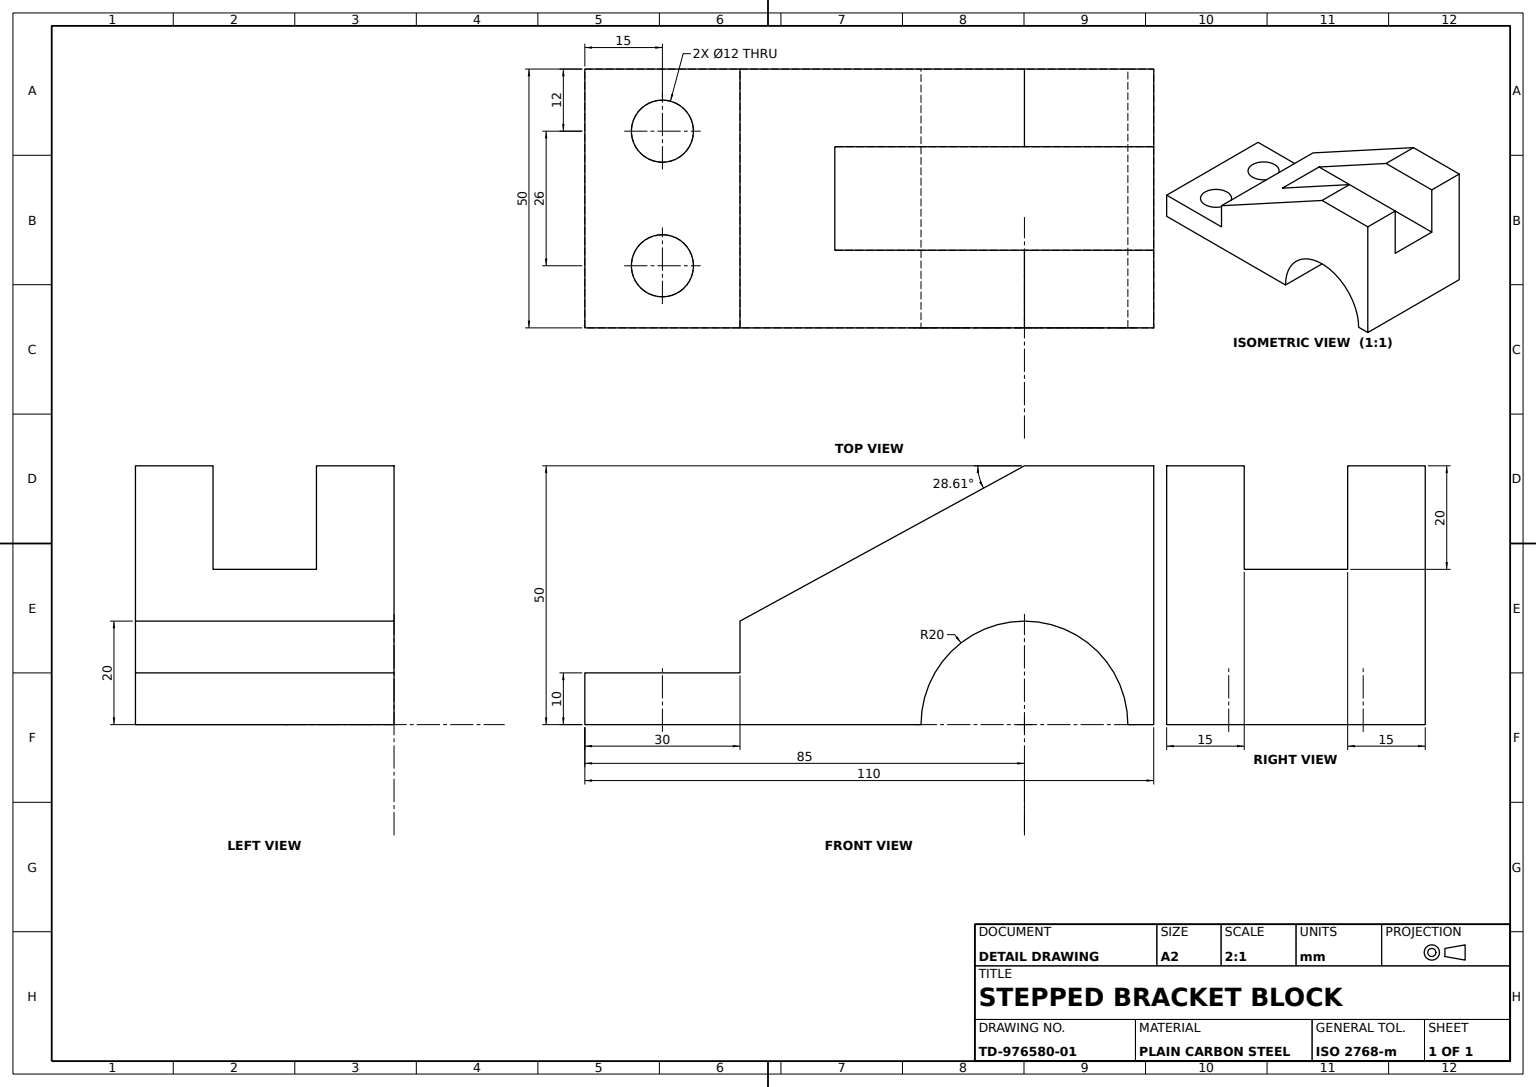
from build123d import *

# Parameters (mm, degrees)
BRACKET_BODY_DEPTH      = 50
TOP_GROOVE_SKETCH_W     = 25
TOP_GROOVE_SKETCH_H     = 20
TOP_GROOVE_CUT_DEPTH    = 20
NOTCH_SKETCH_W          = 20
NOTCH_SKETCH_H          = 20
NOTCH_CUT_DEPTH         = 111.566721937
MOUNTING_HOLES_SKETCH_R = 6
MOUNTING_HOLES_2X_DEPTH = 128.279220614


with BuildPart() as part:
    # Bracket Profile Sketch → Bracket Body (new body)
    with BuildSketch(Plane.XY):
        with BuildLine():
            Line((0, 0), (65, 0))
            ThreePointArc((65, 0), (85, 20), (105, 0))
            Line((105, 0), (110, 0))
            Line((110, 0), (110, 50))
            Line((110, 50), (85, 50))
            Line((85, 50), (30, 20))
            Line((30, 20), (30, 10))
            Line((30, 10), (0, 10))
            Line((0, 10), (0, 0))
        make_face()
    extrude(amount=BRACKET_BODY_DEPTH)

    # Top Groove Sketch → Top Groove Cut (cut)
    with BuildSketch(Plane(origin=(0, 50, 0), x_dir=(1, 0, 0), z_dir=(0, 1, 0))):
        with Locations((97.5, -25)):
            Rectangle(TOP_GROOVE_SKETCH_W, TOP_GROOVE_SKETCH_H)
    extrude(amount=-TOP_GROOVE_CUT_DEPTH, mode=Mode.SUBTRACT)

    # Notch Sketch → Notch Cut (cut, through all)
    with BuildSketch(Plane(origin=(85, 0, 0), x_dir=(0, 0, -1), z_dir=(1, 0, 0))):
        with Locations((-25, 40)):
            Rectangle(NOTCH_SKETCH_W, NOTCH_SKETCH_H)
    extrude(amount=-NOTCH_CUT_DEPTH, mode=Mode.SUBTRACT)

    # Mounting Holes Sketch → Mounting Holes 2x (cut, through all)
    with BuildSketch(Plane(origin=(0, 10, 0), x_dir=(1, 0, 0), z_dir=(0, 1, 0))):
        with Locations(Location((15, -12, 0), (0, 0, 270))):
            Circle(MOUNTING_HOLES_SKETCH_R)
        with Locations(Location((15, -38, 0), (0, 0, 270))):
            Circle(MOUNTING_HOLES_SKETCH_R)
    extrude(amount=-MOUNTING_HOLES_2X_DEPTH, mode=Mode.SUBTRACT)


solid = part.part
